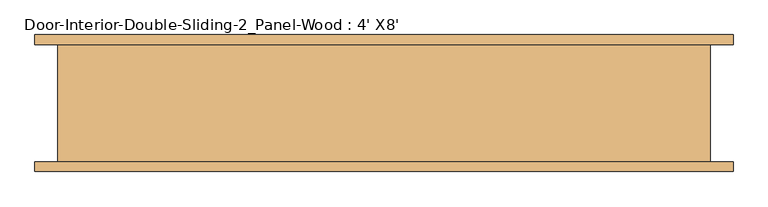
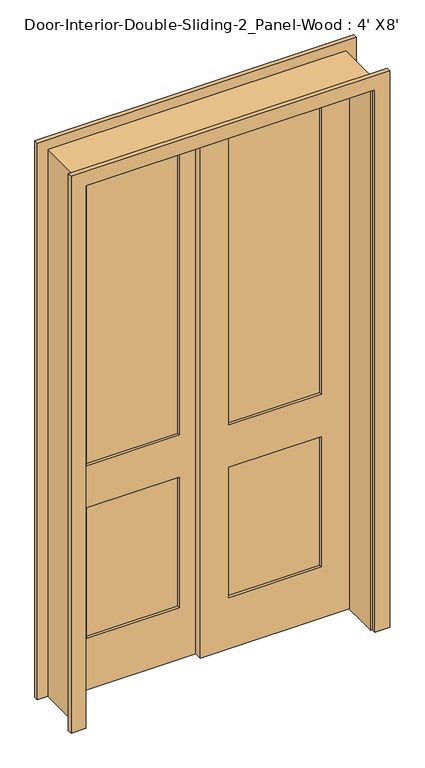
"""IFC4 building model written with IfcOpenShell, lengths in millimetres: door geometry, Door-Interior-Double-Sliding-2_Panel-Wood : 4' X8'."""

from ifc_helpers import new_model, si_unit, frame, origin, place, context, project, spatial, polyline, outline, extrude, source, transform, mapped, element, save


def door_interior_double_sliding_2_panel_wood_4_x8_84ebb68c(model_context):
    return source(origin(), model_context, "Body", "SweptSolid", [
        extrude(outline(polyline([(0.0, 609.6), (0.0, 635.0), (2463.8, 635.0), (2463.8, -635.0), (0.0, -635.0), (0.0, -609.6), (2438.4, -609.6), (2438.4, 609.6), (0.0, 609.6)])), frame((0.0, -117.475, 0.0), z_axis=(0.0, 1.0, 0.0), x_axis=(0.0, 0.0, 1.0)), (0.0, 0.0, 1.0), 228.6),
        extrude(outline(polyline([(2438.4, -609.6), (0.0, -609.6), (0.0, 25.4), (2438.4, 25.4), (2438.4, -609.6)]), holes=[polyline([(2319.3375, -488.95), (2319.3375, -95.25), (1009.65, -95.25), (1009.65, -488.95), (2319.3375, -488.95)]), polyline([(819.15, -488.95), (819.15, -95.25), (231.775, -95.25), (231.775, -488.95), (819.15, -488.95)])]), frame((0.0, 76.2, 0.0), z_axis=(0.0, 1.0, 0.0), x_axis=(0.0, 0.0, 1.0)), (0.0, 0.0, 1.0), 34.925),
        extrude(outline(polyline([(-95.25, 87.8416667), (-488.95, 87.8416667), (-488.95, 99.4833333), (-95.25, 99.4833333), (-95.25, 87.8416667)])), frame((0.0, 0.0, 1009.65), z_axis=(0.0, 0.0, 1.0), x_axis=(1.0, 0.0, 0.0)), (0.0, 0.0, 1.0), 1309.6875),
        extrude(outline(polyline([(-95.25, 87.8416667), (-488.95, 87.8416667), (-488.95, 99.4833333), (-95.25, 99.4833333), (-95.25, 87.8416667)])), frame((0.0, 0.0, 231.775), z_axis=(0.0, 0.0, 1.0), x_axis=(1.0, 0.0, 0.0)), (0.0, 0.0, 1.0), 587.375),
        extrude(outline(polyline([(2438.4, -25.4), (0.0, -25.4), (0.0, 609.6), (2438.4, 609.6), (2438.4, -25.4)]), holes=[polyline([(2319.3375, 95.25), (2319.3375, 488.95), (1009.65, 488.95), (1009.65, 95.25), (2319.3375, 95.25)]), polyline([(819.15, 95.25), (819.15, 488.95), (231.775, 488.95), (231.775, 95.25), (819.15, 95.25)])]), frame((0.0, 41.275, 0.0), z_axis=(0.0, 1.0, 0.0), x_axis=(0.0, 0.0, 1.0)), (0.0, 0.0, 1.0), 34.925),
        extrude(outline(polyline([(488.95, 52.9166667), (95.25, 52.9166667), (95.25, 64.5583333), (488.95, 64.5583333), (488.95, 52.9166667)])), frame((0.0, 0.0, 1009.65), z_axis=(0.0, 0.0, 1.0), x_axis=(1.0, 0.0, 0.0)), (0.0, 0.0, 1.0), 1309.6875),
        extrude(outline(polyline([(488.95, 52.9166667), (95.25, 52.9166667), (95.25, 64.5583333), (488.95, 64.5583333), (488.95, 52.9166667)])), frame((0.0, 0.0, 231.775), z_axis=(0.0, 0.0, 1.0), x_axis=(1.0, 0.0, 0.0)), (0.0, 0.0, 1.0), 587.375),
        extrude(outline(polyline([(0.0, 615.95), (0.0, 679.45), (2508.25, 679.45), (2508.25, -679.45), (0.0, -679.45), (0.0, -615.95), (2444.75, -615.95), (2444.75, 615.95), (0.0, 615.95)])), frame((0.0, 111.125, 0.0), z_axis=(0.0, 1.0, 0.0), x_axis=(0.0, 0.0, 1.0)), (0.0, 0.0, 1.0), 19.05),
        extrude(outline(polyline([(0.0, 615.95), (0.0, 679.45), (2508.25, 679.45), (2508.25, -679.45), (0.0, -679.45), (0.0, -615.95), (2444.75, -615.95), (2444.75, 615.95), (0.0, 615.95)])), frame((0.0, -136.525, 0.0), z_axis=(0.0, 1.0, 0.0), x_axis=(0.0, 0.0, 1.0)), (0.0, 0.0, 1.0), 19.05),
    ])


if __name__ == "__main__":
    model = new_model("IFC4")
    model_context = context("Model", 3, world=origin())
    ifc_project = project(units=[si_unit("LENGTHUNIT", "METRE", prefix="MILLI")], contexts=[model_context])
    site = spatial("IfcSite", under=ifc_project)
    building = spatial("IfcBuilding", under=site)
    placement = place(None, origin())
    door_interior_double_sliding_2_panel_wood_4_x8_shape = door_interior_double_sliding_2_panel_wood_4_x8_84ebb68c(model_context)
    element("IfcDoor", 1, ObjectType="Door-Interior-Double-Sliding-2_Panel-Wood : 4' X8'", at=placement, inside=building, context=model_context, shape_type="MappedRepresentation", body=[
        mapped(door_interior_double_sliding_2_panel_wood_4_x8_shape, transform((0.0, 0.0, 0.0), x_axis=(1.0, 0.0, 0.0), y_axis=(0.0, 1.0, 0.0), z_axis=(0.0, 0.0, 1.0))),
    ])
    save(model, "model.ifc")

# Revit data of these elements
# Type "Door-Interior-Double-Sliding-2_Panel-Wood : 4' X8'"
#   Type Mark = "13"
#   Assembly Code = "C1020300"
#   Analytic Construction = "Wooden"
#   Top Rail = 0' - 4 11/16"
#   Thickness = 0' - 1 3/8"
#   Thermal Resistance (R) = 2.5876 (h·ft²·°F)/BTU
#   Stiles = 0' - 4 3/4"
#   Rough Width = 4' - 2"
#   Rough Height = 8' - 1"
#   Lock Rail = 0' - 7 1/2"
#   Height = 8' - 0"
#   Width = 4' - 0"
#   Heat Transfer Coefficient (U) = 0.3865 BTU/(h·ft²·°F)
#   Bottom Rail = 0' - 9 1/8"
#   Trim Material = Cherry
#   Panel Material = Cherry
#   Frame Material = Cherry
#   Visual Light Transmittance = 0
#   Solar Heat Gain Coefficient = 0
#   Wall Closure = (empty or 0)
#   Function = (empty or 0)
# Element 1 (IfcDoor, "Door-Interior-Double-Sliding-2_Panel-Wood : 4' X8'")
#   Materials on its faces: "Cherry"
# Materials
#   "Cherry": class "Wood", colour RGB 226 177 128, transparency 0, Description = "Prunus Serotina", Cost = 0
